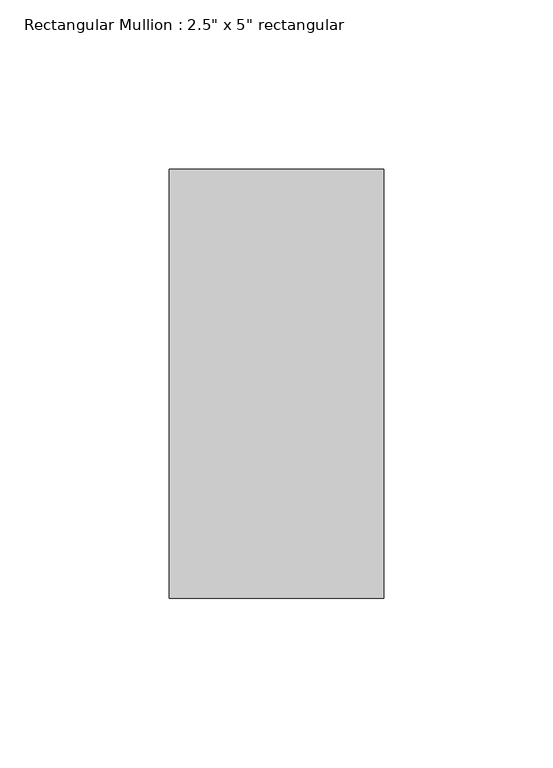
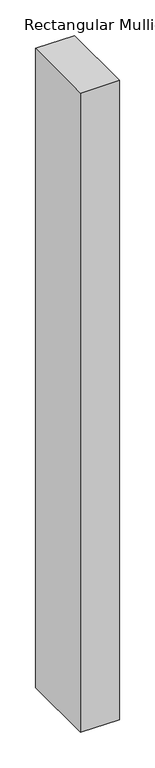
"""IFC4 building model written with IfcOpenShell, lengths in millimetres: member geometry."""

from ifc_helpers import new_model, si_unit, frame, origin, place, context, project, spatial, polyline, outline, extrude, source, transform, mapped, element, save


def member_37269937(model_context):
    return source(origin(), model_context, "Body", "SweptSolid", [
        extrude(outline(polyline([(0.0, 63.5), (0.0, -63.5), (-63.5, -63.5), (-63.5, 63.5), (0.0, 63.5)])), frame((0.0, 0.0, -1098.5500001), z_axis=(0.0, 0.0, 1.0), x_axis=(1.0, 0.0, 0.0)), (0.0, 0.0, 1.0), 1098.5500001),
    ])


if __name__ == "__main__":
    model = new_model("IFC4")
    model_context = context("Model", 3, world=origin())
    ifc_project = project(units=[si_unit("LENGTHUNIT", "METRE", prefix="MILLI")], contexts=[model_context])
    site = spatial("IfcSite", under=ifc_project)
    building = spatial("IfcBuilding", under=site)
    placement = place(None, origin())
    member_shape = member_37269937(model_context)
    element("IfcMember", 1, ObjectType="Rectangular Mullion : 2.5\" x 5\" rectangular", at=placement, inside=building, context=model_context, shape_type="MappedRepresentation", body=[
        mapped(member_shape, transform((0.0, 0.0, 0.0), x_axis=(1.0, 0.0, 0.0), y_axis=(0.0, 1.0, 0.0), z_axis=(0.0, 0.0, 1.0))),
    ])
    save(model, "model.ifc")

# Revit data of these elements
# Type "Rectangular Mullion : 2.5\" x 5\" rectangular"
#   built-in parameter 1007304 = 0.416667 (stored number, unit not read)
#   built-in parameter 1007301 = 0.104167 (stored number, unit not read)
#   built-in parameter 1007300 = 0.104167 (stored number, unit not read)
# Element 1 (IfcMember, "Rectangular Mullion : 2.5\" x 5\" rectangular")
#   Materials on its faces: "BLACK COLOUR"
# Materials
#   "BLACK COLOUR": class "Generic", colour RGB 120 120 120, transparency 0, Cost = 0
